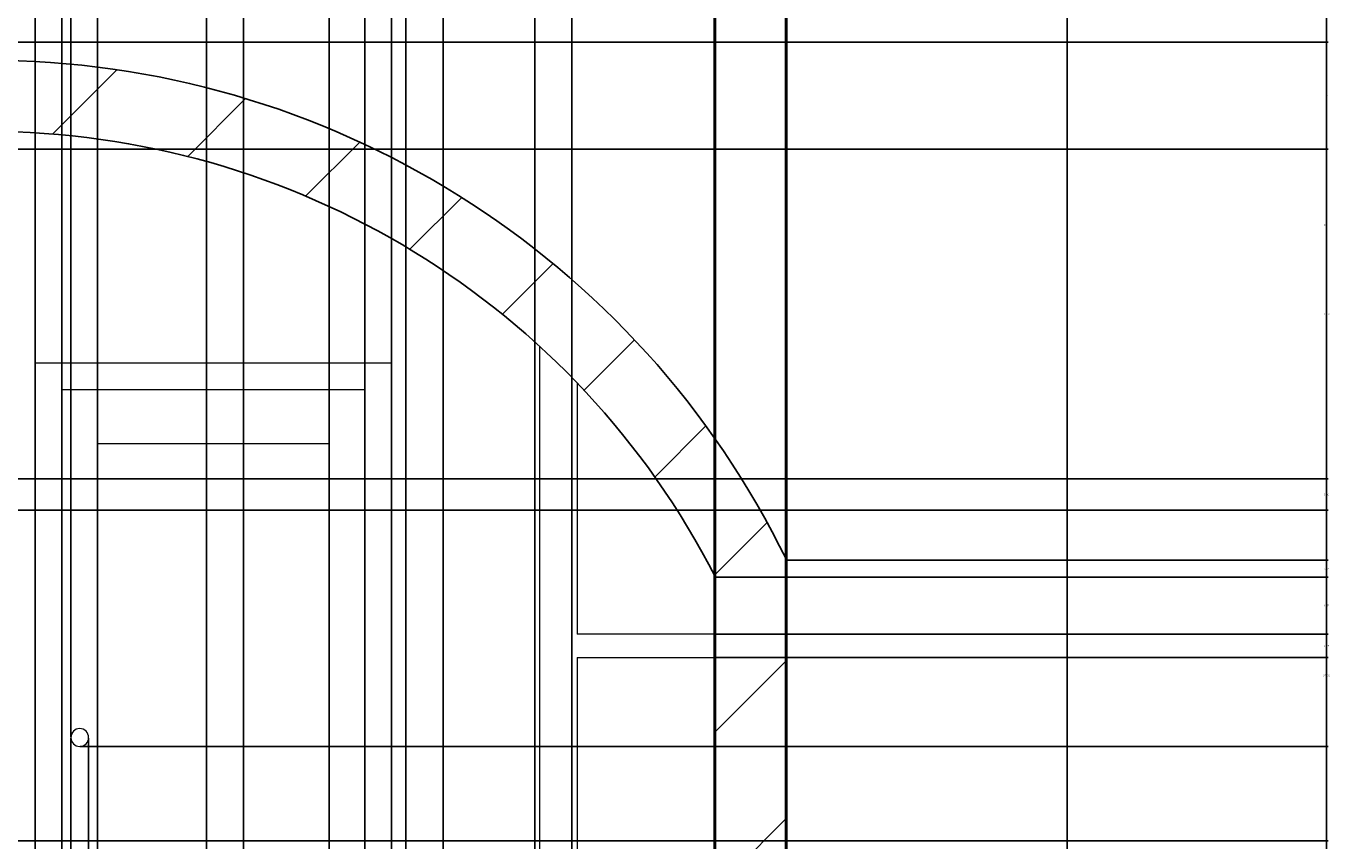
# Model space of a CAD drawing. Units: inches. Extents: x -14 to 375, y -86 to 549.
# Tile 8 of 12: x 228 to 375, y 156 to 248. Entities that reach past the tile are written whole.
import ezdxf

# ---------------------------------------------------------------- set-up
doc = ezdxf.new("R2010")
doc.units = ezdxf.units.IN
doc.header["$MEASUREMENT"] = 0
for name, color, linetype, lineweight in [('A-ANNO-DIMS', 2, 'Continuous', 18), ('A-DOOR', 3, 'Continuous', 18), ('A-ELEV', 7, 'Continuous', 25), ('A-ELEV-PATT', 8, 'Continuous', 13), ('A-GLAZ', 4, 'Continuous', 18)]:
    doc.layers.add(name, color=color, linetype=linetype, lineweight=lineweight)
doc.styles.get("Standard").update_dxf_attribs({"font": 'arial.ttf'})
doc.dimstyles.get("Standard").update_dxf_attribs({"dimtxt": 0.18, "dimasz": 0.18, "dimexe": 0.18, "dimexo": 0.0625, "dimgap": 0.09, "dimtad": 0, "dimtih": 1, "dimtoh": 1, "dimdec": 4, "dimzin": 0, "dimdsep": 46, "dimtxsty": 'Standard', "dimcen": 0.09, "dimadec": 0, "dimazin": 0, "dimtfac": 1, "dimtdec": 4, "dimtofl": 0, "dimtmove": 0, "dimatfit": 3, "dimfxl": 1, "dimtolj": 1, "dimtzin": 0, "dimarcsym": 0})

# ---------------------------------------------------------------- blocks, each defined once
blk = doc.blocks.new('*U3')
blk.add_lwpolyline([(3.12, 0.01), (0.12, 0.01), (0.12, 84.01), (40.12, 84.01), (40.12, 0.01), (37.12, 0.01)])
for points in [[(37.12, 80.99), (37.12, 0.01), (3.12, 0.01), (3.12, 80.99)], [(33.12, 6.01), (33.12, 74.99), (7.12, 74.99), (7.12, 6.01)]]:
    blk.add_lwpolyline(points, close=True)
blk.add_circle((35.12, 42.01), 1)
blk = doc.blocks.new('*D10')
at = {"layer": 'A-ANNO-DIMS', "color": 0, "lineweight": -2, "transparency": 16777216}
for p, q in [((301.52, 485.96), (374.54, 485.96)), ((374.36, 485.78), (374.36, 225.61)), ((374.36, -34.93), (374.36, 225.24)), ((345.33, -35.11), (374.54, -35.11))]:
    blk.add_line(p, q, dxfattribs=at)
at = {"layer": 'A-ANNO-DIMS', "color": 0, "transparency": 16777216}
for points in [[(374.33, 485.78), (374.39, 485.78), (374.36, 485.96)], [(374.33, -34.93), (374.39, -34.93), (374.36, -35.11)]]:
    blk.add_solid(points, dxfattribs=at)
at = {"layer": 'Defpoints', "color": 0, "transparency": 16777216}
for p in [(301.46, 485.96), (374.36, 485.96), (345.26, -35.11)]:
    blk.add_point(p, dxfattribs=at)
at = {"layer": 'A-ANNO-DIMS', "color": 0, "transparency": 16777216, "insert": (374.36, 225.42), "char_height": 0.18, "attachment_point": 5}
blk.add_mtext('\\A1;521.1', dxfattribs=at)
blk = doc.blocks.new('*D29')
at = {"layer": 'A-ANNO-DIMS', "color": 0, "lineweight": -2, "transparency": 16777216}
for p, q in [((107.74, 193.48), (374.54, 193.48)), ((374.36, 193.3), (374.36, 175.11)), ((374.36, 156.56), (374.36, 174.75)), ((107.76, 156.38), (374.54, 156.38))]:
    blk.add_line(p, q, dxfattribs=at)
at = {"layer": 'A-ANNO-DIMS', "color": 0, "transparency": 16777216}
for points in [[(374.33, 193.3), (374.39, 193.3), (374.36, 193.48)], [(374.33, 156.56), (374.39, 156.56), (374.36, 156.38)]]:
    blk.add_solid(points, dxfattribs=at)
at = {"layer": 'Defpoints', "color": 0, "transparency": 16777216}
for p in [(107.68, 193.48), (374.36, 193.48), (107.7, 156.38)]:
    blk.add_point(p, dxfattribs=at)
at = {"layer": 'A-ANNO-DIMS', "color": 0, "transparency": 16777216, "insert": (374.36, 174.93), "char_height": 0.18, "attachment_point": 5}
blk.add_mtext('\\A1;37.106', dxfattribs=at)
blk = doc.blocks.new('*D30')
at = {"layer": 'A-ANNO-DIMS', "color": 0, "lineweight": -2, "transparency": 16777216}
for p, q in [((107.74, 196.98), (374.54, 196.98)), ((374.36, 196.8), (374.36, 195.41)), ((374.36, 193.66), (374.36, 195.05)), ((107.74, 193.48), (374.54, 193.48))]:
    blk.add_line(p, q, dxfattribs=at)
at = {"layer": 'A-ANNO-DIMS', "color": 0, "transparency": 16777216}
for points in [[(374.33, 196.8), (374.39, 196.8), (374.36, 196.98)], [(374.33, 193.66), (374.39, 193.66), (374.36, 193.48)]]:
    blk.add_solid(points, dxfattribs=at)
at = {"layer": 'Defpoints', "color": 0, "transparency": 16777216}
for p in [(107.68, 196.98), (374.36, 196.98), (107.68, 193.48)]:
    blk.add_point(p, dxfattribs=at)
at = {"layer": 'A-ANNO-DIMS', "color": 0, "transparency": 16777216, "insert": (374.36, 195.23), "char_height": 0.18, "attachment_point": 5}
blk.add_mtext('\\A1;3.501', dxfattribs=at)
blk = doc.blocks.new('*D31')
at = {"layer": 'A-ANNO-DIMS', "color": 0, "lineweight": -2, "transparency": 16777216}
for p, q in [((107.76, 233.96), (374.54, 233.96)), ((374.36, 233.78), (374.36, 215.65)), ((374.36, 197.16), (374.36, 215.29)), ((107.74, 196.98), (374.54, 196.98))]:
    blk.add_line(p, q, dxfattribs=at)
at = {"layer": 'A-ANNO-DIMS', "color": 0, "transparency": 16777216}
for points in [[(374.33, 233.78), (374.39, 233.78), (374.36, 233.96)], [(374.33, 197.16), (374.39, 197.16), (374.36, 196.98)]]:
    blk.add_solid(points, dxfattribs=at)
at = {"layer": 'Defpoints', "color": 0, "transparency": 16777216}
for p in [(107.7, 233.96), (374.36, 233.96), (107.68, 196.98)]:
    blk.add_point(p, dxfattribs=at)
at = {"layer": 'A-ANNO-DIMS', "color": 0, "transparency": 16777216, "insert": (374.36, 215.47), "char_height": 0.18, "attachment_point": 5}
blk.add_mtext('\\A1;36.975', dxfattribs=at)
blk = doc.blocks.new('*D32')
at = {"layer": 'A-ANNO-DIMS', "color": 0, "lineweight": -2, "transparency": 16777216}
for p, q in [((107.76, 245.96), (374.54, 245.96)), ((374.36, 245.78), (374.36, 240.14)), ((374.36, 234.14), (374.36, 239.78)), ((107.76, 233.96), (374.54, 233.96))]:
    blk.add_line(p, q, dxfattribs=at)
at = {"layer": 'A-ANNO-DIMS', "color": 0, "transparency": 16777216}
for points in [[(374.33, 245.78), (374.39, 245.78), (374.36, 245.96)], [(374.33, 234.14), (374.39, 234.14), (374.36, 233.96)]]:
    blk.add_solid(points, dxfattribs=at)
at = {"layer": 'Defpoints', "color": 0, "transparency": 16777216}
for p in [(107.7, 245.96), (374.36, 245.96), (107.7, 233.96)]:
    blk.add_point(p, dxfattribs=at)
at = {"layer": 'A-ANNO-DIMS', "color": 0, "transparency": 16777216, "insert": (374.36, 239.96), "char_height": 0.18, "attachment_point": 5}
blk.add_mtext('\\A1;12', dxfattribs=at)
blk = doc.blocks.new('*D33')
at = {"layer": 'A-ANNO-DIMS', "color": 0, "lineweight": -2, "transparency": 16777216}
for p, q in [((107.76, 254.96), (374.54, 254.96)), ((374.36, 254.78), (374.36, 250.64)), ((374.36, 246.14), (374.36, 250.28)), ((107.76, 245.96), (374.54, 245.96))]:
    blk.add_line(p, q, dxfattribs=at)
at = {"layer": 'A-ANNO-DIMS', "color": 0, "transparency": 16777216}
for points in [[(374.33, 254.78), (374.39, 254.78), (374.36, 254.96)], [(374.33, 246.14), (374.39, 246.14), (374.36, 245.96)]]:
    blk.add_solid(points, dxfattribs=at)
at = {"layer": 'Defpoints', "color": 0, "transparency": 16777216}
for p in [(107.7, 254.96), (374.36, 254.96), (107.7, 245.96)]:
    blk.add_point(p, dxfattribs=at)
at = {"layer": 'A-ANNO-DIMS', "color": 0, "transparency": 16777216, "insert": (374.36, 250.46), "char_height": 0.18, "attachment_point": 5}
blk.add_mtext('\\A1;9', dxfattribs=at)
blk = doc.blocks.new('*D43')
at = {"layer": 'A-ANNO-DIMS', "color": 0, "lineweight": -2, "transparency": 16777216}
for p, q in [((142.23, 270.64), (142.23, -64.39)), ((305.63, 270.64), (305.63, -64.39)), ((142.41, -64.21), (223.55, -64.21)), ((305.45, -64.21), (224.32, -64.21))]:
    blk.add_line(p, q, dxfattribs=at)
at = {"layer": 'A-ANNO-DIMS', "color": 0, "transparency": 16777216}
for points in [[(142.41, -64.18), (142.41, -64.24), (142.23, -64.21)], [(305.45, -64.18), (305.45, -64.24), (305.63, -64.21)]]:
    blk.add_solid(points, dxfattribs=at)
at = {"layer": 'Defpoints', "color": 0, "transparency": 16777216}
for p in [(142.23, 270.71), (305.63, 270.71), (305.63, -64.21)]:
    blk.add_point(p, dxfattribs=at)
at = {"layer": 'A-ANNO-DIMS', "color": 0, "transparency": 16777216, "insert": (223.93, -64.21), "char_height": 0.18, "attachment_point": 5}
blk.add_mtext('\\A1;163.4', dxfattribs=at)
blk = doc.blocks.new('*D44')
at = {"layer": 'A-ANNO-DIMS', "color": 0, "lineweight": -2, "transparency": 16777216}
for p, q in [((305.63, 270.64), (305.63, -64.39)), ((313.63, 262.64), (313.63, -64.39)), ((305.81, -64.21), (309.48, -64.21)), ((313.45, -64.21), (309.78, -64.21))]:
    blk.add_line(p, q, dxfattribs=at)
at = {"layer": 'A-ANNO-DIMS', "color": 0, "transparency": 16777216}
for points in [[(305.81, -64.18), (305.81, -64.24), (305.63, -64.21)], [(313.45, -64.18), (313.45, -64.24), (313.63, -64.21)]]:
    blk.add_solid(points, dxfattribs=at)
at = {"layer": 'Defpoints', "color": 0, "transparency": 16777216}
for p in [(305.63, 270.71), (313.63, 262.71), (313.63, -64.21)]:
    blk.add_point(p, dxfattribs=at)
at = {"layer": 'A-ANNO-DIMS', "color": 0, "transparency": 16777216, "insert": (309.63, -64.21), "char_height": 0.18, "attachment_point": 5}
blk.add_mtext('\\A1;8', dxfattribs=at)
blk = doc.blocks.new('*D49')
at = {"layer": 'A-ANNO-DIMS', "color": 0, "lineweight": -2, "transparency": 16777216}
for p, q in [((215.95, 306.64), (215.95, -64.39)), ((248.64, 306.64), (248.64, -64.39)), ((216.13, -64.21), (231.9, -64.21)), ((248.46, -64.21), (232.69, -64.21))]:
    blk.add_line(p, q, dxfattribs=at)
at = {"layer": 'A-ANNO-DIMS', "color": 0, "transparency": 16777216}
for points in [[(216.13, -64.18), (216.13, -64.24), (215.95, -64.21)], [(248.46, -64.18), (248.46, -64.24), (248.64, -64.21)]]:
    blk.add_solid(points, dxfattribs=at)
at = {"layer": 'Defpoints', "color": 0, "transparency": 16777216}
for p in [(215.95, 306.71), (248.64, 306.71), (248.64, -64.21)]:
    blk.add_point(p, dxfattribs=at)
at = {"layer": 'A-ANNO-DIMS', "color": 0, "transparency": 16777216, "insert": (232.29, -64.21), "char_height": 0.18, "attachment_point": 5}
blk.add_mtext('\\A1;32.69', dxfattribs=at)
blk = doc.blocks.new('*D50')
at = {"layer": 'A-ANNO-DIMS', "color": 0, "lineweight": -2, "transparency": 16777216}
for p, q in [((248.64, 306.64), (248.64, -64.39)), ((252.81, 306.64), (252.81, -64.39)), ((248.82, -64.21), (250.39, -64.21)), ((252.63, -64.21), (251.05, -64.21))]:
    blk.add_line(p, q, dxfattribs=at)
at = {"layer": 'A-ANNO-DIMS', "color": 0, "transparency": 16777216}
for points in [[(248.82, -64.18), (248.82, -64.24), (248.64, -64.21)], [(252.63, -64.18), (252.63, -64.24), (252.81, -64.21)]]:
    blk.add_solid(points, dxfattribs=at)
at = {"layer": 'Defpoints', "color": 0, "transparency": 16777216}
for p in [(248.64, 306.71), (252.81, 306.71), (252.81, -64.21)]:
    blk.add_point(p, dxfattribs=at)
at = {"layer": 'A-ANNO-DIMS', "color": 0, "transparency": 16777216, "insert": (250.72, -64.21), "char_height": 0.18, "attachment_point": 5}
blk.add_mtext('\\A1;4.17', dxfattribs=at)
blk = doc.blocks.new('*D51')
at = {"layer": 'A-ANNO-DIMS', "color": 0, "lineweight": -2, "transparency": 16777216}
for p, q in [((252.81, 306.64), (252.81, -64.39)), ((285.5, 306.64), (285.5, -64.39)), ((252.99, -64.21), (268.76, -64.21)), ((285.32, -64.21), (269.54, -64.21))]:
    blk.add_line(p, q, dxfattribs=at)
at = {"layer": 'A-ANNO-DIMS', "color": 0, "transparency": 16777216}
for points in [[(252.99, -64.18), (252.99, -64.24), (252.81, -64.21)], [(285.32, -64.18), (285.32, -64.24), (285.5, -64.21)]]:
    blk.add_solid(points, dxfattribs=at)
at = {"layer": 'Defpoints', "color": 0, "transparency": 16777216}
for p in [(252.81, 306.71), (285.5, 306.71), (285.5, -64.21)]:
    blk.add_point(p, dxfattribs=at)
at = {"layer": 'A-ANNO-DIMS', "color": 0, "transparency": 16777216, "insert": (269.15, -64.21), "char_height": 0.18, "attachment_point": 5}
blk.add_mtext('\\A1;32.69', dxfattribs=at)
blk = doc.blocks.new('*D52')
at = {"layer": 'A-ANNO-DIMS', "color": 0, "lineweight": -2, "transparency": 16777216}
for p, q in [((285.5, 306.64), (285.5, -64.39)), ((289.66, 306.64), (289.66, -64.39)), ((285.68, -64.21), (287.25, -64.21)), ((289.48, -64.21), (287.91, -64.21))]:
    blk.add_line(p, q, dxfattribs=at)
at = {"layer": 'A-ANNO-DIMS', "color": 0, "transparency": 16777216}
for points in [[(285.68, -64.18), (285.68, -64.24), (285.5, -64.21)], [(289.48, -64.18), (289.48, -64.24), (289.66, -64.21)]]:
    blk.add_solid(points, dxfattribs=at)
at = {"layer": 'Defpoints', "color": 0, "transparency": 16777216}
for p in [(285.5, 306.71), (289.66, 306.71), (289.66, -64.21)]:
    blk.add_point(p, dxfattribs=at)
at = {"layer": 'A-ANNO-DIMS', "color": 0, "transparency": 16777216, "insert": (287.58, -64.21), "char_height": 0.18, "attachment_point": 5}
blk.add_mtext('\\A1;4.17', dxfattribs=at)
blk = doc.blocks.new('*D57')
at = {"layer": 'A-ANNO-DIMS', "color": 0, "lineweight": -2, "transparency": 16777216}
for p, q in [((229.41, 340.38), (229.41, -64.39)), ((232.41, 340.38), (232.41, -64.39)), ((229.59, -64.21), (230.76, -64.21)), ((232.23, -64.21), (231.06, -64.21))]:
    blk.add_line(p, q, dxfattribs=at)
at = {"layer": 'A-ANNO-DIMS', "color": 0, "transparency": 16777216}
for points in [[(229.59, -64.18), (229.59, -64.24), (229.41, -64.21)], [(232.23, -64.18), (232.23, -64.24), (232.41, -64.21)]]:
    blk.add_solid(points, dxfattribs=at)
at = {"layer": 'Defpoints', "color": 0, "transparency": 16777216}
for p in [(229.41, 340.44), (232.41, 340.44), (232.41, -64.21)]:
    blk.add_point(p, dxfattribs=at)
at = {"layer": 'A-ANNO-DIMS', "color": 0, "transparency": 16777216, "insert": (230.91, -64.21), "char_height": 0.18, "attachment_point": 5}
blk.add_mtext('\\A1;3', dxfattribs=at)
blk = doc.blocks.new('*D58')
at = {"layer": 'A-ANNO-DIMS', "color": 0, "lineweight": -2, "transparency": 16777216}
for p, q in [((232.41, 340.38), (232.41, -64.39)), ((236.41, 340.38), (236.41, -64.39)), ((232.59, -64.21), (234.26, -64.21)), ((236.23, -64.21), (234.56, -64.21))]:
    blk.add_line(p, q, dxfattribs=at)
at = {"layer": 'A-ANNO-DIMS', "color": 0, "transparency": 16777216}
for points in [[(232.59, -64.18), (232.59, -64.24), (232.41, -64.21)], [(236.23, -64.18), (236.23, -64.24), (236.41, -64.21)]]:
    blk.add_solid(points, dxfattribs=at)
at = {"layer": 'Defpoints', "color": 0, "transparency": 16777216}
for p in [(232.41, 340.44), (236.41, 340.44), (236.41, -64.21)]:
    blk.add_point(p, dxfattribs=at)
at = {"layer": 'A-ANNO-DIMS', "color": 0, "transparency": 16777216, "insert": (234.41, -64.21), "char_height": 0.18, "attachment_point": 5}
blk.add_mtext('\\A1;4', dxfattribs=at)
blk = doc.blocks.new('*D59')
at = {"layer": 'A-ANNO-DIMS', "color": 0, "lineweight": -2, "transparency": 16777216}
for p, q in [((236.41, 340.38), (236.41, -64.39)), ((262.41, 340.38), (262.41, -64.39)), ((236.59, -64.21), (249.19, -64.21)), ((262.23, -64.21), (249.63, -64.21))]:
    blk.add_line(p, q, dxfattribs=at)
at = {"layer": 'A-ANNO-DIMS', "color": 0, "transparency": 16777216}
for points in [[(236.59, -64.18), (236.59, -64.24), (236.41, -64.21)], [(262.23, -64.18), (262.23, -64.24), (262.41, -64.21)]]:
    blk.add_solid(points, dxfattribs=at)
at = {"layer": 'Defpoints', "color": 0, "transparency": 16777216}
for p in [(236.41, 340.44), (262.41, 340.44), (262.41, -64.21)]:
    blk.add_point(p, dxfattribs=at)
at = {"layer": 'A-ANNO-DIMS', "color": 0, "transparency": 16777216, "insert": (249.41, -64.21), "char_height": 0.18, "attachment_point": 5}
blk.add_mtext('\\A1;26', dxfattribs=at)
blk = doc.blocks.new('*D60')
at = {"layer": 'A-ANNO-DIMS', "color": 0, "lineweight": -2, "transparency": 16777216}
for p, q in [((262.41, 340.38), (262.41, -64.39)), ((266.41, 340.38), (266.41, -64.39)), ((262.59, -64.21), (264.26, -64.21)), ((266.23, -64.21), (264.56, -64.21))]:
    blk.add_line(p, q, dxfattribs=at)
at = {"layer": 'A-ANNO-DIMS', "color": 0, "transparency": 16777216}
for points in [[(262.59, -64.18), (262.59, -64.24), (262.41, -64.21)], [(266.23, -64.18), (266.23, -64.24), (266.41, -64.21)]]:
    blk.add_solid(points, dxfattribs=at)
at = {"layer": 'Defpoints', "color": 0, "transparency": 16777216}
for p in [(262.41, 340.44), (266.41, 340.44), (266.41, -64.21)]:
    blk.add_point(p, dxfattribs=at)
at = {"layer": 'A-ANNO-DIMS', "color": 0, "transparency": 16777216, "insert": (264.41, -64.21), "char_height": 0.18, "attachment_point": 5}
blk.add_mtext('\\A1;4', dxfattribs=at)
blk = doc.blocks.new('*D61')
at = {"layer": 'A-ANNO-DIMS', "color": 0, "lineweight": -2, "transparency": 16777216}
for p, q in [((266.41, 340.38), (266.41, -64.39)), ((269.41, 340.38), (269.41, -64.39)), ((266.59, -64.21), (267.76, -64.21)), ((269.23, -64.21), (268.06, -64.21))]:
    blk.add_line(p, q, dxfattribs=at)
at = {"layer": 'A-ANNO-DIMS', "color": 0, "transparency": 16777216}
for points in [[(266.59, -64.18), (266.59, -64.24), (266.41, -64.21)], [(269.23, -64.18), (269.23, -64.24), (269.41, -64.21)]]:
    blk.add_solid(points, dxfattribs=at)
at = {"layer": 'Defpoints', "color": 0, "transparency": 16777216}
for p in [(266.41, 340.44), (269.41, 340.44), (269.41, -64.21)]:
    blk.add_point(p, dxfattribs=at)
at = {"layer": 'A-ANNO-DIMS', "color": 0, "transparency": 16777216, "insert": (267.91, -64.21), "char_height": 0.18, "attachment_point": 5}
blk.add_mtext('\\A1;3', dxfattribs=at)
blk = doc.blocks.new('*D71')
at = {"layer": 'A-ANNO-DIMS', "color": 0, "lineweight": -2, "transparency": 16777216}
for p, q in [((233.41, 167.91), (233.41, -64.39)), ((235.41, 167.91), (235.41, -64.39)), ((233.59, -64.21), (234.26, -64.21)), ((235.23, -64.21), (234.56, -64.21))]:
    blk.add_line(p, q, dxfattribs=at)
at = {"layer": 'A-ANNO-DIMS', "color": 0, "transparency": 16777216}
for points in [[(233.59, -64.18), (233.59, -64.24), (233.41, -64.21)], [(235.23, -64.18), (235.23, -64.24), (235.41, -64.21)]]:
    blk.add_solid(points, dxfattribs=at)
at = {"layer": 'Defpoints', "color": 0, "transparency": 16777216}
for p in [(233.41, 167.97), (235.41, 167.97), (235.41, -64.21)]:
    blk.add_point(p, dxfattribs=at)
at = {"layer": 'A-ANNO-DIMS', "color": 0, "transparency": 16777216, "insert": (234.41, -64.21), "char_height": 0.18, "attachment_point": 5}
blk.add_mtext('\\A1;2', dxfattribs=at)
blk = doc.blocks.new('*D72')
at = {"layer": 'A-ANNO-DIMS', "color": 0, "lineweight": -2, "transparency": 16777216}
for p, q in [((229.41, 126.03), (229.41, 515.24)), ((233.41, 168.03), (233.41, 515.24)), ((229.59, 515.06), (231.26, 515.06)), ((233.23, 515.06), (231.56, 515.06))]:
    blk.add_line(p, q, dxfattribs=at)
at = {"layer": 'A-ANNO-DIMS', "color": 0, "transparency": 16777216}
for points in [[(229.59, 515.09), (229.59, 515.03), (229.41, 515.06)], [(233.23, 515.09), (233.23, 515.03), (233.41, 515.06)]]:
    blk.add_solid(points, dxfattribs=at)
at = {"layer": 'Defpoints', "color": 0, "transparency": 16777216}
for p in [(233.41, 515.06), (233.41, 167.97), (229.41, 125.97)]:
    blk.add_point(p, dxfattribs=at)
at = {"layer": 'A-ANNO-DIMS', "color": 0, "transparency": 16777216, "insert": (231.41, 515.06), "char_height": 0.18, "attachment_point": 5}
blk.add_mtext('\\A1;4', dxfattribs=at)
blk = doc.blocks.new('*D73')
at = {"layer": 'A-ANNO-DIMS', "color": 0, "lineweight": -2, "transparency": 16777216}
for p, q in [((234.47, 166.97), (374.54, 166.97)), ((374.36, 166.79), (374.36, 146.65)), ((374.36, 126.15), (374.36, 146.29)), ((269.47, 125.97), (374.54, 125.97))]:
    blk.add_line(p, q, dxfattribs=at)
at = {"layer": 'A-ANNO-DIMS', "color": 0, "transparency": 16777216}
for points in [[(374.33, 166.79), (374.39, 166.79), (374.36, 166.97)], [(374.33, 126.15), (374.39, 126.15), (374.36, 125.97)]]:
    blk.add_solid(points, dxfattribs=at)
at = {"layer": 'Defpoints', "color": 0, "transparency": 16777216}
for p in [(234.41, 166.97), (374.36, 166.97), (269.41, 125.97)]:
    blk.add_point(p, dxfattribs=at)
at = {"layer": 'A-ANNO-DIMS', "color": 0, "transparency": 16777216, "insert": (374.36, 146.47), "char_height": 0.18, "attachment_point": 5}
blk.add_mtext('\\A1;41', dxfattribs=at)
blk = doc.blocks.new('*D85')
at = {"layer": 'A-ANNO-DIMS', "color": 0, "lineweight": -2, "transparency": 16777216}
for p, q in [((229.41, 210.03), (229.41, 515.24)), ((232.41, 207.01), (232.41, 515.24)), ((229.59, 515.06), (230.76, 515.06)), ((232.23, 515.06), (231.06, 515.06))]:
    blk.add_line(p, q, dxfattribs=at)
at = {"layer": 'A-ANNO-DIMS', "color": 0, "transparency": 16777216}
for points in [[(229.59, 515.09), (229.59, 515.03), (229.41, 515.06)], [(232.23, 515.09), (232.23, 515.03), (232.41, 515.06)]]:
    blk.add_solid(points, dxfattribs=at)
at = {"layer": 'Defpoints', "color": 0, "transparency": 16777216}
for p in [(232.41, 515.06), (229.41, 209.97), (232.41, 206.95)]:
    blk.add_point(p, dxfattribs=at)
at = {"layer": 'A-ANNO-DIMS', "color": 0, "transparency": 16777216, "insert": (230.91, 515.06), "char_height": 0.18, "attachment_point": 5}
blk.add_mtext('\\A1;3', dxfattribs=at)
blk = doc.blocks.new('*D86')
at = {"layer": 'A-ANNO-DIMS', "color": 0, "lineweight": -2, "transparency": 16777216}
for p, q in [((232.41, 207.01), (232.41, 515.24)), ((236.41, 201.01), (236.41, 515.24)), ((232.59, 515.06), (234.26, 515.06)), ((236.23, 515.06), (234.56, 515.06))]:
    blk.add_line(p, q, dxfattribs=at)
at = {"layer": 'A-ANNO-DIMS', "color": 0, "transparency": 16777216}
for points in [[(232.59, 515.09), (232.59, 515.03), (232.41, 515.06)], [(236.23, 515.09), (236.23, 515.03), (236.41, 515.06)]]:
    blk.add_solid(points, dxfattribs=at)
at = {"layer": 'Defpoints', "color": 0, "transparency": 16777216}
for p in [(236.41, 515.06), (232.41, 206.95), (236.41, 200.95)]:
    blk.add_point(p, dxfattribs=at)
at = {"layer": 'A-ANNO-DIMS', "color": 0, "transparency": 16777216, "insert": (234.41, 515.06), "char_height": 0.18, "attachment_point": 5}
blk.add_mtext('\\A1;4', dxfattribs=at)
blk = doc.blocks.new('*D87')
at = {"layer": 'A-ANNO-DIMS', "color": 0, "lineweight": -2, "transparency": 16777216}
for p, q in [((236.41, 201.01), (236.41, 515.24)), ((262.41, 201.01), (262.41, 515.24)), ((236.59, 515.06), (249.19, 515.06)), ((262.23, 515.06), (249.63, 515.06))]:
    blk.add_line(p, q, dxfattribs=at)
at = {"layer": 'A-ANNO-DIMS', "color": 0, "transparency": 16777216}
for points in [[(236.59, 515.09), (236.59, 515.03), (236.41, 515.06)], [(262.23, 515.09), (262.23, 515.03), (262.41, 515.06)]]:
    blk.add_solid(points, dxfattribs=at)
at = {"layer": 'Defpoints', "color": 0, "transparency": 16777216}
for p in [(262.41, 515.06), (236.41, 200.95), (262.41, 200.95)]:
    blk.add_point(p, dxfattribs=at)
at = {"layer": 'A-ANNO-DIMS', "color": 0, "transparency": 16777216, "insert": (249.41, 515.06), "char_height": 0.18, "attachment_point": 5}
blk.add_mtext('\\A1;26', dxfattribs=at)
blk = doc.blocks.new('*D88')
at = {"layer": 'A-ANNO-DIMS', "color": 0, "lineweight": -2, "transparency": 16777216}
for p, q in [((262.41, 201.01), (262.41, 515.24)), ((266.41, 207.01), (266.41, 515.24)), ((262.59, 515.06), (264.26, 515.06)), ((266.23, 515.06), (264.56, 515.06))]:
    blk.add_line(p, q, dxfattribs=at)
at = {"layer": 'A-ANNO-DIMS', "color": 0, "transparency": 16777216}
for points in [[(262.59, 515.09), (262.59, 515.03), (262.41, 515.06)], [(266.23, 515.09), (266.23, 515.03), (266.41, 515.06)]]:
    blk.add_solid(points, dxfattribs=at)
at = {"layer": 'Defpoints', "color": 0, "transparency": 16777216}
for p in [(266.41, 515.06), (266.41, 206.95), (262.41, 200.95)]:
    blk.add_point(p, dxfattribs=at)
at = {"layer": 'A-ANNO-DIMS', "color": 0, "transparency": 16777216, "insert": (264.41, 515.06), "char_height": 0.18, "attachment_point": 5}
blk.add_mtext('\\A1;4', dxfattribs=at)
blk = doc.blocks.new('*D89')
at = {"layer": 'A-ANNO-DIMS', "color": 0, "lineweight": -2, "transparency": 16777216}
for p, q in [((266.41, 207.01), (266.41, 515.24)), ((269.41, 210.03), (269.41, 515.24)), ((266.59, 515.06), (267.76, 515.06)), ((269.23, 515.06), (268.06, 515.06))]:
    blk.add_line(p, q, dxfattribs=at)
at = {"layer": 'A-ANNO-DIMS', "color": 0, "transparency": 16777216}
for points in [[(266.59, 515.09), (266.59, 515.03), (266.41, 515.06)], [(269.23, 515.09), (269.23, 515.03), (269.41, 515.06)]]:
    blk.add_solid(points, dxfattribs=at)
at = {"layer": 'Defpoints', "color": 0, "transparency": 16777216}
for p in [(269.41, 515.06), (269.41, 209.97), (266.41, 206.95)]:
    blk.add_point(p, dxfattribs=at)
at = {"layer": 'A-ANNO-DIMS', "color": 0, "transparency": 16777216, "insert": (267.91, 515.06), "char_height": 0.18, "attachment_point": 5}
blk.add_mtext('\\A1;3', dxfattribs=at)
blk = doc.blocks.new('*D91')
at = {"layer": 'A-ANNO-DIMS', "color": 0, "lineweight": -2, "transparency": 16777216}
for p, q in [((305.83, 176.93), (374.54, 176.93)), ((374.36, 176.75), (374.36, 151.63)), ((374.36, 126.14), (374.36, 151.26)), ((305.83, 125.96), (374.54, 125.96))]:
    blk.add_line(p, q, dxfattribs=at)
at = {"layer": 'A-ANNO-DIMS', "color": 0, "transparency": 16777216}
for points in [[(374.33, 176.75), (374.39, 176.75), (374.36, 176.93)], [(374.33, 126.14), (374.39, 126.14), (374.36, 125.96)]]:
    blk.add_solid(points, dxfattribs=at)
at = {"layer": 'Defpoints', "color": 0, "transparency": 16777216}
for p in [(305.77, 176.93), (374.36, 176.93), (305.77, 125.96)]:
    blk.add_point(p, dxfattribs=at)
at = {"layer": 'A-ANNO-DIMS', "color": 0, "transparency": 16777216, "insert": (374.36, 151.45), "char_height": 0.18, "attachment_point": 5}
blk.add_mtext('\\A1;50.97', dxfattribs=at)
blk = doc.blocks.new('*D92')
at = {"layer": 'A-ANNO-DIMS', "color": 0, "lineweight": -2, "transparency": 16777216}
for p, q in [((305.83, 179.58), (374.54, 179.58)), ((374.36, 179.4), (374.36, 178.44)), ((374.36, 177.11), (374.36, 178.07)), ((305.83, 176.93), (374.54, 176.93))]:
    blk.add_line(p, q, dxfattribs=at)
at = {"layer": 'A-ANNO-DIMS', "color": 0, "transparency": 16777216}
for points in [[(374.33, 179.4), (374.39, 179.4), (374.36, 179.58)], [(374.33, 177.11), (374.39, 177.11), (374.36, 176.93)]]:
    blk.add_solid(points, dxfattribs=at)
at = {"layer": 'Defpoints', "color": 0, "transparency": 16777216}
for p in [(305.77, 179.58), (374.36, 179.58), (305.77, 176.93)]:
    blk.add_point(p, dxfattribs=at)
at = {"layer": 'A-ANNO-DIMS', "color": 0, "transparency": 16777216, "insert": (374.36, 178.26), "char_height": 0.18, "attachment_point": 5}
blk.add_mtext('\\A1;2.649', dxfattribs=at)
blk = doc.blocks.new('*D93')
at = {"layer": 'A-ANNO-DIMS', "color": 0, "lineweight": -2, "transparency": 16777216}
for p, q in [((305.83, 185.96), (374.54, 185.96)), ((374.36, 185.78), (374.36, 182.95)), ((374.36, 179.76), (374.36, 182.59)), ((305.83, 179.58), (374.54, 179.58))]:
    blk.add_line(p, q, dxfattribs=at)
at = {"layer": 'A-ANNO-DIMS', "color": 0, "transparency": 16777216}
for points in [[(374.33, 185.78), (374.39, 185.78), (374.36, 185.96)], [(374.33, 179.76), (374.39, 179.76), (374.36, 179.58)]]:
    blk.add_solid(points, dxfattribs=at)
at = {"layer": 'Defpoints', "color": 0, "transparency": 16777216}
for p in [(305.77, 185.96), (374.36, 185.96), (305.77, 179.58)]:
    blk.add_point(p, dxfattribs=at)
at = {"layer": 'A-ANNO-DIMS', "color": 0, "transparency": 16777216, "insert": (374.36, 182.77), "char_height": 0.18, "attachment_point": 5}
blk.add_mtext('\\A1;6.378', dxfattribs=at)
blk = doc.blocks.new('*D94')
at = {"layer": 'A-ANNO-DIMS', "color": 0, "lineweight": -2, "transparency": 16777216}
for p, q in [((313.83, 187.85), (374.54, 187.85)), ((374.36, 187.67), (374.36, 187.08)), ((305.83, 185.96), (374.54, 185.96)), ((374.36, 186.14), (374.36, 186.72))]:
    blk.add_line(p, q, dxfattribs=at)
at = {"layer": 'A-ANNO-DIMS', "color": 0, "transparency": 16777216}
for points in [[(374.33, 187.67), (374.39, 187.67), (374.36, 187.85)], [(374.33, 186.14), (374.39, 186.14), (374.36, 185.96)]]:
    blk.add_solid(points, dxfattribs=at)
at = {"layer": 'Defpoints', "color": 0, "transparency": 16777216}
for p in [(313.77, 187.85), (374.36, 187.85), (305.77, 185.96)]:
    blk.add_point(p, dxfattribs=at)
at = {"layer": 'A-ANNO-DIMS', "color": 0, "transparency": 16777216, "insert": (374.36, 186.9), "char_height": 0.18, "attachment_point": 5}
blk.add_mtext('\\A1;1.89', dxfattribs=at)
blk = doc.blocks.new('*D104')
at = {"layer": 'A-ANNO-DIMS', "color": 0, "lineweight": -2, "transparency": 16777216}
for p, q in [((190.15, 6.02), (190.15, 515.24)), ((271, 6.02), (271, 515.24)), ((190.33, 515.06), (230.18, 515.06)), ((270.82, 515.06), (230.97, 515.06))]:
    blk.add_line(p, q, dxfattribs=at)
at = {"layer": 'A-ANNO-DIMS', "color": 0, "transparency": 16777216}
for points in [[(190.33, 515.09), (190.33, 515.03), (190.15, 515.06)], [(270.82, 515.09), (270.82, 515.03), (271, 515.06)]]:
    blk.add_solid(points, dxfattribs=at)
at = {"layer": 'Defpoints', "color": 0, "transparency": 16777216}
for p in [(271, 515.06), (190.15, 5.96), (271, 5.96)]:
    blk.add_point(p, dxfattribs=at)
at = {"layer": 'A-ANNO-DIMS', "color": 0, "transparency": 16777216, "insert": (230.57, 515.06), "char_height": 0.18, "attachment_point": 5}
blk.add_mtext('\\A1;80.85', dxfattribs=at)
blk = doc.blocks.new('*D105')
at = {"layer": 'A-ANNO-DIMS', "color": 0, "lineweight": -2, "transparency": 16777216}
for p, q in [((271, 6.02), (271, 515.24)), ((275.19, 6.02), (275.19, 515.24)), ((271.18, 515.06), (272.69, 515.06)), ((275.01, 515.06), (273.49, 515.06))]:
    blk.add_line(p, q, dxfattribs=at)
at = {"layer": 'A-ANNO-DIMS', "color": 0, "transparency": 16777216}
for points in [[(271.18, 515.09), (271.18, 515.03), (271, 515.06)], [(275.01, 515.09), (275.01, 515.03), (275.19, 515.06)]]:
    blk.add_solid(points, dxfattribs=at)
at = {"layer": 'Defpoints', "color": 0, "transparency": 16777216}
for p in [(275.19, 515.06), (271, 5.96), (275.19, 5.96)]:
    blk.add_point(p, dxfattribs=at)
at = {"layer": 'A-ANNO-DIMS', "color": 0, "transparency": 16777216, "insert": (273.09, 515.06), "char_height": 0.18, "attachment_point": 5}
blk.add_mtext('\\A1;4.186', dxfattribs=at)
blk = doc.blocks.new('*D106')
at = {"layer": 'A-ANNO-DIMS', "color": 0, "lineweight": -2, "transparency": 16777216}
for p, q in [((275.19, 6.02), (275.19, 515.24)), ((305.77, 6.02), (305.77, 515.24)), ((275.37, 515.06), (290.01, 515.06)), ((305.59, 515.06), (290.94, 515.06))]:
    blk.add_line(p, q, dxfattribs=at)
at = {"layer": 'A-ANNO-DIMS', "color": 0, "transparency": 16777216}
for points in [[(275.37, 515.09), (275.37, 515.03), (275.19, 515.06)], [(305.59, 515.09), (305.59, 515.03), (305.77, 515.06)]]:
    blk.add_solid(points, dxfattribs=at)
at = {"layer": 'Defpoints', "color": 0, "transparency": 16777216}
for p in [(305.77, 515.06), (275.19, 5.96), (305.77, 5.96)]:
    blk.add_point(p, dxfattribs=at)
at = {"layer": 'A-ANNO-DIMS', "color": 0, "transparency": 16777216, "insert": (290.48, 515.06), "char_height": 0.18, "attachment_point": 5}
blk.add_mtext('\\A1;30.585', dxfattribs=at)
blk = doc.blocks.new('*D107')
at = {"layer": 'A-ANNO-DIMS', "color": 0, "lineweight": -2, "transparency": 16777216}
for p, q in [((305.77, 6.02), (305.77, 515.24)), ((313.77, 6.02), (313.77, 515.24)), ((305.95, 515.06), (309.62, 515.06)), ((313.59, 515.06), (309.92, 515.06))]:
    blk.add_line(p, q, dxfattribs=at)
at = {"layer": 'A-ANNO-DIMS', "color": 0, "transparency": 16777216}
for points in [[(305.95, 515.09), (305.95, 515.03), (305.77, 515.06)], [(313.59, 515.09), (313.59, 515.03), (313.77, 515.06)]]:
    blk.add_solid(points, dxfattribs=at)
at = {"layer": 'Defpoints', "color": 0, "transparency": 16777216}
for p in [(313.77, 515.06), (305.77, 5.96), (313.77, 5.96)]:
    blk.add_point(p, dxfattribs=at)
at = {"layer": 'A-ANNO-DIMS', "color": 0, "transparency": 16777216, "insert": (309.77, 515.06), "char_height": 0.18, "attachment_point": 5}
blk.add_mtext('\\A1;8', dxfattribs=at)

msp = doc.modelspace()

# ---------------------------------------------------------------- hatches: boundary and pattern name
at = {"layer": 'A-ELEV-PATT'}
h = msp.add_hatch(dxfattribs=at)
h.set_pattern_fill('ANSI31', color=256, scale=100)
h.set_pattern_definition([(45, (-168.406, -22.703), (-8.83883, 8.83883), [])])
h.paths.add_polyline_path([(313.6281, 262.7071), (313.6281, 357.9589), (313.7701, 357.9589), (313.7701, 433.1717, 0.36940998), (134.2334, 433.1717), (134.2334, 365.9589), (134.2334, 262.7071)])
h.paths.add_polyline_path([(142.2334, 270.7071), (142.2334, 365.9589), (142.2334, 429.4208, -0.35358711), (305.7701, 429.4208), (305.7701, 365.9589), (305.6281, 365.9589), (305.6281, 270.7071)], flags=16)
h.paths.add_polyline_path([(134.2334, 187.8466), (134.2334, 117.9589), (313.7701, 117.9589), (313.7701, 187.8466, 0.62486768)])
h.paths.add_polyline_path([(305.7701, 185.9589), (305.7701, 125.9589), (142.2334, 125.9589), (142.2334, 185.9589, -0.61125102)], flags=16)
h.paths.add_polyline_path([(134.2334, 73.1717), (134.2334, 5.9589), (142.2334, 5.9589), (142.2334, 69.4208, -0.35358711), (305.7701, 69.4208), (305.7701, 5.9589), (313.7701, 5.9589), (313.7701, 73.1717, 0.36940998)])

# ---------------------------------------------------------------- linework, layer by layer
at = {"layer": 'A-ELEV'}
msp.add_lwpolyline([(345.2647, 5.9589), (345.2647, 125.9589), (345.2647, 245.9589), (345.2647, 365.9589), (345.2647, 442.1495, 0.41421356), (301.4553, 485.9589)], format="xyb", dxfattribs=at)
for points in [[(134.2334, 187.8466), (134.2334, 117.9589), (313.7701, 117.9589), (313.7701, 187.8466, 0.62486768)], [(142.2334, 185.9589), (142.2334, 125.9589), (305.7701, 125.9589), (305.7701, 185.9589, 0.61125102)]]:
    msp.add_lwpolyline(points, format="xyb", close=True, dxfattribs=at)
at = {"layer": 'A-GLAZ'}
for points in [[(290.2356, 176.9318), (290.2356, 125.9589), (286.0499, 125.9589), (286.0499, 211.8227)], [(286.0499, 179.5807), (286.0499, 211.8227)], [(290.2356, 207.7373), (290.2356, 179.5807)], [(290.2356, 176.9318), (305.7701, 176.9318), (305.7701, 179.5807), (290.2356, 179.5807)]]:
    msp.add_lwpolyline(points, dxfattribs=at)

# ---------------------------------------------------------------- block references
at = {"layer": 'A-DOOR', "xscale": -1}
msp.add_blockref('*U3', (269.5328, 125.9589), dxfattribs=at)

# ---------------------------------------------------------------- dimensions: what is measured, and where the dimension line sits
at = {"layer": 'A-ANNO-DIMS'}
for base, p1, p2, override, picture, middle in [((270.9993, 515.0589), (190.148, 5.9589), (270.9993, 5.9589), {"dimdec": 2, "dimlfac": 1, "dimrnd": 0, "dimzin": 0, "dimdsep": 46, "dimlunit": 2}, '*D104', (230.5736, 515.0589)), ((233.409, 515.0589), (229.409, 125.9717), (233.409, 167.9717), {"dimdec": 0, "dimlfac": 1, "dimrnd": 0, "dimzin": 0, "dimdsep": 46, "dimlunit": 2}, '*D72', (231.409, 515.0589)), ((232.409, 515.0589), (229.409, 209.9717), (232.409, 206.9487), {"dimdec": 0, "dimlfac": 1, "dimrnd": 0, "dimzin": 0, "dimdsep": 46, "dimlunit": 2}, '*D85', (230.909, 515.0589)), ((236.409, 515.0589), (232.409, 206.9487), (236.409, 200.9487), {"dimdec": 0, "dimlfac": 1, "dimrnd": 0, "dimzin": 0, "dimdsep": 46, "dimlunit": 2}, '*D86', (234.409, 515.0589)), ((262.409, 515.0589), (236.409, 200.9487), (262.409, 200.9487), {"dimdec": 0, "dimlfac": 1, "dimrnd": 0, "dimzin": 0, "dimdsep": 46, "dimlunit": 2}, '*D87', (249.409, 515.0589)), ((266.409, 515.0589), (262.409, 200.9487), (266.409, 206.9487), {"dimdec": 0, "dimlfac": 1, "dimrnd": 0, "dimzin": 0, "dimdsep": 46, "dimlunit": 2}, '*D88', (264.409, 515.0589)), ((269.409, 515.0589), (266.409, 206.9487), (269.409, 209.9717), {"dimdec": 0, "dimlfac": 1, "dimrnd": 0, "dimzin": 0, "dimdsep": 46, "dimlunit": 2}, '*D89', (267.909, 515.0589)), ((275.185, 515.0589), (270.9993, 5.9589), (275.185, 5.9589), {"dimdec": 3, "dimlfac": 1, "dimrnd": 0, "dimzin": 0, "dimdsep": 46, "dimlunit": 2}, '*D105', (273.0921, 515.0589)), ((305.7701, 515.0589), (275.185, 5.9589), (305.7701, 5.9589), {"dimdec": 3, "dimlfac": 1, "dimrnd": 0, "dimzin": 0, "dimdsep": 46, "dimlunit": 2}, '*D106', (290.4775, 515.0589)), ((313.7701, 515.0589), (305.7701, 5.9589), (313.7701, 5.9589), {"dimdec": 0, "dimlfac": 1, "dimrnd": 0, "dimzin": 0, "dimdsep": 46, "dimlunit": 2}, '*D107', (309.7701, 515.0589)), ((232.409, -64.2115), (229.409, 340.4421), (232.409, 340.4421), {"dimdec": 0, "dimlfac": 1, "dimrnd": 0, "dimzin": 0, "dimdsep": 46, "dimlunit": 2}, '*D57', (230.909, -64.2115)), ((236.409, -64.2115), (232.409, 340.4421), (236.409, 340.4421), {"dimdec": 0, "dimlfac": 1, "dimrnd": 0, "dimzin": 0, "dimdsep": 46, "dimlunit": 2}, '*D58', (234.409, -64.2115)), ((262.409, -64.2115), (236.409, 340.4421), (262.409, 340.4421), {"dimdec": 0, "dimlfac": 1, "dimrnd": 0, "dimzin": 0, "dimdsep": 46, "dimlunit": 2}, '*D59', (249.409, -64.2115)), ((266.409, -64.2115), (262.409, 340.4421), (266.409, 340.4421), {"dimdec": 0, "dimlfac": 1, "dimrnd": 0, "dimzin": 0, "dimdsep": 46, "dimlunit": 2}, '*D60', (264.409, -64.2115)), ((269.409, -64.2115), (266.409, 340.4421), (269.409, 340.4421), {"dimdec": 0, "dimlfac": 1, "dimrnd": 0, "dimzin": 0, "dimdsep": 46, "dimlunit": 2}, '*D61', (267.909, -64.2115)), ((248.639, -64.2115), (215.9481, 306.7071), (248.639, 306.7071), {"dimdec": 2, "dimlfac": 1, "dimrnd": 0, "dimzin": 0, "dimdsep": 46, "dimlunit": 2}, '*D49', (232.2936, -64.2115)), ((252.8055, -64.2115), (248.639, 306.7071), (252.8055, 306.7071), {"dimdec": 2, "dimlfac": 1, "dimrnd": 0, "dimzin": 0, "dimdsep": 46, "dimlunit": 2}, '*D50', (250.7222, -64.2115)), ((285.4964, -64.2115), (252.8055, 306.7071), (285.4964, 306.7071), {"dimdec": 2, "dimlfac": 1, "dimrnd": 0, "dimzin": 0, "dimdsep": 46, "dimlunit": 2}, '*D51', (269.1509, -64.2115)), ((289.6628, -64.2115), (285.4964, 306.7071), (289.6628, 306.7071), {"dimdec": 2, "dimlfac": 1, "dimrnd": 0, "dimzin": 0, "dimdsep": 46, "dimlunit": 2}, '*D52', (287.5796, -64.2115)), ((305.6281, -64.2115), (142.2334, 270.7071), (305.6281, 270.7071), {"dimdec": 1, "dimlfac": 1, "dimrnd": 0, "dimzin": 0, "dimdsep": 46, "dimlunit": 2}, '*D43', (223.9307, -64.2115)), ((313.6281, -64.2115), (305.6281, 270.7071), (313.6281, 262.7071), {"dimdec": 0, "dimlfac": 1, "dimrnd": 0, "dimzin": 0, "dimdsep": 46, "dimlunit": 2}, '*D44', (309.6281, -64.2115)), ((235.409, -64.2115), (233.409, 167.9717), (235.409, 167.9717), {"dimdec": 0, "dimlfac": 1, "dimrnd": 0, "dimzin": 0, "dimdsep": 46, "dimlunit": 2}, '*D71', (234.409, -64.2115))]:
    dim = msp.add_linear_dim(base=base, p1=p1, p2=p2, dimstyle='Standard', override=override, dxfattribs=at)
    dim.commit()
    dim.dimension.update_dxf_attribs({"geometry": picture, "text_midpoint": middle})
for base, p1, p2, override, picture, middle in [((374.3647, 485.9589), (345.2647, -35.1115), (301.4553, 485.9589), {"dimdec": 1, "dimlfac": 1, "dimrnd": 0, "dimzin": 0, "dimdsep": 46, "dimlunit": 2}, '*D10', (374.3647, 225.4237)), ((374.3647, 254.9589), (107.7019, 245.9589), (107.7019, 254.9589), {"dimdec": 0, "dimlfac": 1, "dimrnd": 0, "dimzin": 0, "dimdsep": 46, "dimlunit": 2}, '*D33', (374.3647, 250.4589)), ((374.3647, 245.9589), (107.7019, 233.9589), (107.7019, 245.9589), {"dimdec": 0, "dimlfac": 1, "dimrnd": 0, "dimzin": 0, "dimdsep": 46, "dimlunit": 2}, '*D32', (374.3647, 239.9589)), ((374.3647, 233.9589), (107.6798, 196.9836), (107.7019, 233.9589), {"dimdec": 3, "dimlfac": 1, "dimrnd": 0, "dimzin": 0, "dimdsep": 46, "dimlunit": 2}, '*D31', (374.3647, 215.4712)), ((374.3647, 196.9836), (107.6798, 193.4825), (107.6798, 196.9836), {"dimdec": 3, "dimlfac": 1, "dimrnd": 0, "dimzin": 0, "dimdsep": 46, "dimlunit": 2}, '*D30', (374.3647, 195.233)), ((374.3647, 193.4825), (107.7019, 156.3768), (107.6798, 193.4825), {"dimdec": 3, "dimlfac": 1, "dimrnd": 0, "dimzin": 0, "dimdsep": 46, "dimlunit": 2}, '*D29', (374.3647, 174.9296)), ((374.3647, 187.8466), (305.7701, 185.9589), (313.7701, 187.8466), {"dimdec": 2, "dimlfac": 1, "dimrnd": 0, "dimzin": 0, "dimdsep": 46, "dimlunit": 2}, '*D94', (374.3647, 186.9027)), ((374.3647, 185.9589), (305.7701, 179.5807), (305.7701, 185.9589), {"dimdec": 3, "dimlfac": 1, "dimrnd": 0, "dimzin": 0, "dimdsep": 46, "dimlunit": 2}, '*D93', (374.3647, 182.7698)), ((374.3647, 179.5807), (305.7701, 176.9318), (305.7701, 179.5807), {"dimdec": 3, "dimlfac": 1, "dimrnd": 0, "dimzin": 0, "dimdsep": 46, "dimlunit": 2}, '*D92', (374.3647, 178.2562)), ((374.3647, 176.9318), (305.7701, 125.9589), (305.7701, 176.9318), {"dimdec": 2, "dimlfac": 1, "dimrnd": 0, "dimzin": 0, "dimdsep": 46, "dimlunit": 2}, '*D91', (374.3647, 151.4454)), ((374.3647, 166.9717), (269.409, 125.9717), (234.409, 166.9717), {"dimdec": 0, "dimlfac": 1, "dimrnd": 0, "dimzin": 0, "dimdsep": 46, "dimlunit": 2}, '*D73', (374.3647, 146.4717))]:
    dim = msp.add_linear_dim(base=base, p1=p1, p2=p2, angle=90, dimstyle='Standard', override=override, dxfattribs=at)
    dim.commit()
    dim.dimension.update_dxf_attribs({"geometry": picture, "text_midpoint": middle})

doc.saveas('drawing.dxf')
